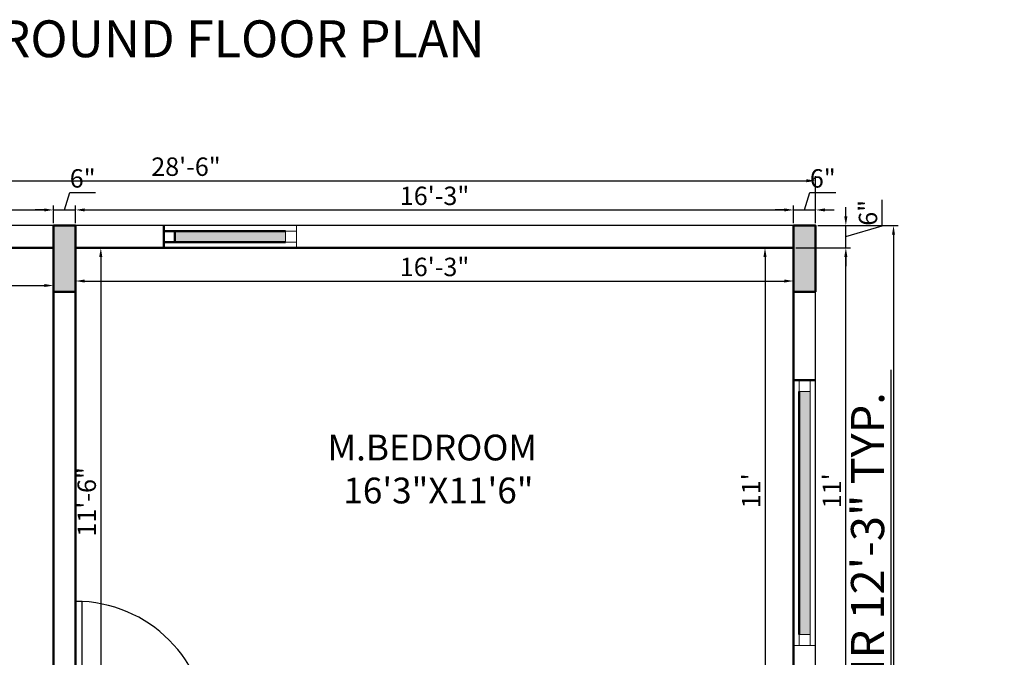
# Model space of a CAD drawing. Units: inches. Extents: x 3064 to 19385, y 846 to 15425.
# Tile 52 of 108: x 6168 to 6436, y 1279 to 1452. Entities that reach past the tile are written whole.
import ezdxf

# ---------------------------------------------------------------- set-up
doc = ezdxf.new("R2010")
doc.units = ezdxf.units.IN
for name, color, linetype, lineweight in [('A-ANNO-DIMS', 2, 'Continuous', 18), ('A-ANNO-TEXT', 7, 'Continuous', 25), ('A-AREA-IDEN', 3, 'Continuous', 18), ('A-COLS', 1, 'Continuous', 35), ('A-DOOR', 3, 'Continuous', 25), ('A-GLAZ', 4, 'Continuous', 18), ('A-WALL', 7, 'Continuous', 50), ('C-PROP', 6, 'Continuous', 25)]:
    doc.layers.add(name, color=color, linetype=linetype, lineweight=lineweight)
doc.styles.get("Standard").update_dxf_attribs({"font": 'arial.ttf'})
doc.dimstyles.new('ISO-25', dxfattribs={"dimtxt": 9, "dimasz": 2.5, "dimexe": 1.25, "dimexo": 0.625, "dimtad": 1, "dimdec": 1, "dimlunit": 3, "dimtxsty": 'Standard', "dimcen": 2.5, "dimadec": 0, "dimazin": 0, "dimtfac": 1, "dimtdec": 1, "dimtmove": 0, "dimatfit": 3, "dimfxl": 1, "dimarcsym": 0})

# ---------------------------------------------------------------- blocks, each defined once
blk = doc.blocks.new('*U3')
for p, q in [((0, 0), (0, -6)), ((36, 0), (36, -6))]:
    blk.add_line(p, q)
blk.add_lwpolyline([(0, 0), (0, 36), (1.75, 36), (1.75, 0)], close=True)
blk.add_arc((0, 0), 36, 0, 90)
blk = doc.blocks.new('*D141')
at = {"layer": 'A-ANNO-DIMS', "color": 0, "lineweight": -2, "transparency": 16777216}
for p, q in [((6048.49, 1396.96), (6048.49, 1401.84)), ((6177.49, 1396.96), (6177.49, 1401.84)), ((6050.99, 1400.59), (6174.99, 1400.59))]:
    blk.add_line(p, q, dxfattribs=at)
at = {"layer": 'A-ANNO-DIMS', "color": 0, "transparency": 16777216}
for points in [[(6050.99, 1401.01), (6050.99, 1400.18), (6048.49, 1400.59)], [(6174.99, 1401.01), (6174.99, 1400.18), (6177.49, 1400.59)]]:
    blk.add_solid(points, dxfattribs=at)
at = {"layer": 'Defpoints', "color": 0, "transparency": 16777216}
for p in [(6177.49, 1400.59), (6048.49, 1396.34), (6177.49, 1396.34)]:
    blk.add_point(p, dxfattribs=at)
at = {"layer": 'A-ANNO-DIMS', "color": 0, "transparency": 16777216, "insert": (6112.99, 1403.77), "char_height": 5, "attachment_point": 5}
blk.add_mtext('10\'-9"', dxfattribs=at)
blk = doc.blocks.new('*D142')
at = {"layer": 'A-ANNO-DIMS', "color": 0, "lineweight": -2, "transparency": 16777216}
for p, q in [((6180.49, 1400.59), (6181.91, 1405.33)), ((6181.91, 1405.33), (6188.94, 1405.33)), ((6177.49, 1396.96), (6177.49, 1401.84)), ((6183.49, 1396.96), (6183.49, 1401.84)), ((6174.99, 1400.59), (6172.49, 1400.59)), ((6177.49, 1400.59), (6183.49, 1400.59)), ((6177.49, 1400.59), (6183.49, 1400.59)), ((6185.99, 1400.59), (6188.49, 1400.59))]:
    blk.add_line(p, q, dxfattribs=at)
at = {"layer": 'A-ANNO-DIMS', "color": 0, "transparency": 16777216}
for points in [[(6174.99, 1401.01), (6174.99, 1400.18), (6177.49, 1400.59)], [(6185.99, 1401.01), (6185.99, 1400.18), (6183.49, 1400.59)]]:
    blk.add_solid(points, dxfattribs=at)
at = {"layer": 'Defpoints', "color": 0, "transparency": 16777216}
for p in [(6183.49, 1400.59), (6177.49, 1396.34), (6183.49, 1396.34)]:
    blk.add_point(p, dxfattribs=at)
at = {"layer": 'A-ANNO-DIMS', "color": 0, "transparency": 16777216, "insert": (6185.43, 1408.51), "char_height": 5, "attachment_point": 5}
blk.add_mtext('6"', dxfattribs=at)
blk = doc.blocks.new('*D143')
at = {"layer": 'A-ANNO-DIMS', "color": 0, "lineweight": -2, "transparency": 16777216}
for p, q in [((6183.49, 1396.96), (6183.49, 1401.84)), ((6378.49, 1396.96), (6378.49, 1401.84)), ((6185.99, 1400.59), (6375.99, 1400.59))]:
    blk.add_line(p, q, dxfattribs=at)
at = {"layer": 'A-ANNO-DIMS', "color": 0, "transparency": 16777216}
for points in [[(6185.99, 1401.01), (6185.99, 1400.18), (6183.49, 1400.59)], [(6375.99, 1401.01), (6375.99, 1400.18), (6378.49, 1400.59)]]:
    blk.add_solid(points, dxfattribs=at)
at = {"layer": 'Defpoints', "color": 0, "transparency": 16777216}
for p in [(6378.49, 1400.59), (6183.49, 1396.34), (6378.49, 1396.34)]:
    blk.add_point(p, dxfattribs=at)
at = {"layer": 'A-ANNO-DIMS', "color": 0, "transparency": 16777216, "insert": (6280.99, 1403.77), "char_height": 5, "attachment_point": 5}
blk.add_mtext('16\'-3"', dxfattribs=at)
blk = doc.blocks.new('*D144')
at = {"layer": 'A-ANNO-DIMS', "color": 0, "lineweight": -2, "transparency": 16777216}
for p, q in [((6381.49, 1400.59), (6382.91, 1405.33)), ((6382.91, 1405.33), (6389.94, 1405.33)), ((6378.49, 1396.96), (6378.49, 1401.84)), ((6384.49, 1396.96), (6384.49, 1401.84)), ((6375.99, 1400.59), (6373.49, 1400.59)), ((6378.49, 1400.59), (6384.49, 1400.59)), ((6378.49, 1400.59), (6384.49, 1400.59)), ((6386.99, 1400.59), (6389.49, 1400.59))]:
    blk.add_line(p, q, dxfattribs=at)
at = {"layer": 'A-ANNO-DIMS', "color": 0, "transparency": 16777216}
for points in [[(6375.99, 1401.01), (6375.99, 1400.18), (6378.49, 1400.59)], [(6386.99, 1401.01), (6386.99, 1400.18), (6384.49, 1400.59)]]:
    blk.add_solid(points, dxfattribs=at)
at = {"layer": 'Defpoints', "color": 0, "transparency": 16777216}
for p in [(6384.49, 1400.59), (6378.49, 1396.34), (6384.49, 1396.34)]:
    blk.add_point(p, dxfattribs=at)
at = {"layer": 'A-ANNO-DIMS', "color": 0, "transparency": 16777216, "insert": (6386.43, 1408.51), "char_height": 5, "attachment_point": 5}
blk.add_mtext('6"', dxfattribs=at)
blk = doc.blocks.new('*D131')
at = {"layer": 'A-ANNO-DIMS', "color": 0, "lineweight": -2, "transparency": 16777216}
for p, q in [((6379.12, 1390.34), (6393.94, 1390.34)), ((6392.69, 1260.84), (6392.69, 1387.84)), ((6385.12, 1258.34), (6393.94, 1258.34))]:
    blk.add_line(p, q, dxfattribs=at)
at = {"layer": 'A-ANNO-DIMS', "color": 0, "transparency": 16777216}
for points in [[(6392.27, 1387.84), (6393.1, 1387.84), (6392.69, 1390.34)], [(6392.27, 1260.84), (6393.1, 1260.84), (6392.69, 1258.34)]]:
    blk.add_solid(points, dxfattribs=at)
at = {"layer": 'Defpoints', "color": 0, "transparency": 16777216}
for p in [(6378.49, 1390.34), (6392.69, 1390.34), (6384.49, 1258.34)]:
    blk.add_point(p, dxfattribs=at)
at = {"layer": 'A-ANNO-DIMS', "color": 0, "transparency": 16777216, "insert": (6389.55, 1324.34), "char_height": 5, "attachment_point": 5, "rotation": 90}
blk.add_mtext("11'", dxfattribs=at)
blk = doc.blocks.new('*D132')
at = {"layer": 'A-ANNO-DIMS', "color": 0, "lineweight": -2, "transparency": 16777216}
for p, q in [((6392.69, 1398.84), (6392.69, 1401.34)), ((6402.53, 1396.29), (6402.53, 1403.32)), ((6385.12, 1396.34), (6393.94, 1396.34)), ((6392.69, 1390.34), (6392.69, 1396.34)), ((6392.69, 1390.34), (6392.69, 1396.34)), ((6392.69, 1393.34), (6402.53, 1396.29)), ((6379.12, 1390.34), (6393.94, 1390.34)), ((6392.69, 1387.84), (6392.69, 1385.34))]:
    blk.add_line(p, q, dxfattribs=at)
at = {"layer": 'A-ANNO-DIMS', "color": 0, "transparency": 16777216}
for points in [[(6392.27, 1398.84), (6393.1, 1398.84), (6392.69, 1396.34)], [(6392.27, 1387.84), (6393.1, 1387.84), (6392.69, 1390.34)]]:
    blk.add_solid(points, dxfattribs=at)
at = {"layer": 'Defpoints', "color": 0, "transparency": 16777216}
for p in [(6384.49, 1396.34), (6392.69, 1396.34), (6378.49, 1390.34)]:
    blk.add_point(p, dxfattribs=at)
at = {"layer": 'A-ANNO-DIMS', "color": 0, "transparency": 16777216, "insert": (6399.35, 1399.81), "char_height": 5, "attachment_point": 5, "rotation": 90}
blk.add_mtext('6"', dxfattribs=at)
blk = doc.blocks.new('*D133')
at = {"layer": 'A-ANNO-DIMS', "color": 0, "lineweight": -2, "transparency": 16777216}
for p, q in [((6385.12, 1396.34), (6406.89, 1396.34)), ((6405.64, 1393.84), (6405.64, 882.84)), ((6385.12, 880.34), (6406.89, 880.34))]:
    blk.add_line(p, q, dxfattribs=at)
at = {"layer": 'A-ANNO-DIMS', "color": 0, "transparency": 16777216}
for points in [[(6405.22, 1393.84), (6406.05, 1393.84), (6405.64, 1396.34)], [(6405.22, 882.84), (6406.05, 882.84), (6405.64, 880.34)]]:
    blk.add_solid(points, dxfattribs=at)
at = {"layer": 'Defpoints', "color": 0, "transparency": 16777216}
for p in [(6384.49, 1396.34), (6384.49, 880.34), (6405.64, 880.34)]:
    blk.add_point(p, dxfattribs=at)
at = {"layer": 'A-ANNO-DIMS', "color": 0, "transparency": 16777216, "insert": (6402.46, 1138.34), "char_height": 5, "attachment_point": 5, "rotation": 90}
blk.add_mtext("43'", dxfattribs=at)
blk = doc.blocks.new('*D134')
at = {"layer": 'A-ANNO-DIMS', "color": 0, "lineweight": -2, "transparency": 16777216}
for p, q in [((6042.49, 1396.96), (6042.49, 1409.76)), ((6384.49, 1396.96), (6384.49, 1409.76)), ((6044.99, 1408.51), (6381.99, 1408.51))]:
    blk.add_line(p, q, dxfattribs=at)
at = {"layer": 'A-ANNO-DIMS', "color": 0, "transparency": 16777216}
for points in [[(6044.99, 1408.93), (6044.99, 1408.1), (6042.49, 1408.51)], [(6381.99, 1408.93), (6381.99, 1408.1), (6384.49, 1408.51)]]:
    blk.add_solid(points, dxfattribs=at)
at = {"layer": 'Defpoints', "color": 0, "transparency": 16777216}
for p in [(6384.49, 1408.51), (6042.49, 1396.34), (6384.49, 1396.34)]:
    blk.add_point(p, dxfattribs=at)
at = {"layer": 'A-ANNO-DIMS', "color": 0, "transparency": 16777216, "insert": (6213.49, 1411.69), "char_height": 5, "attachment_point": 5}
blk.add_mtext('28\'-6"', dxfattribs=at)
blk = doc.blocks.new('*D148')
at = {"layer": 'A-ANNO-DIMS', "color": 0, "lineweight": -2, "transparency": 16777216}
for p, q in [((6048.49, 1389.71), (6048.49, 1378.82)), ((6177.49, 1389.71), (6177.49, 1378.82)), ((6050.99, 1380.07), (6174.99, 1380.07))]:
    blk.add_line(p, q, dxfattribs=at)
at = {"layer": 'A-ANNO-DIMS', "color": 0, "transparency": 16777216}
for points in [[(6050.99, 1380.49), (6050.99, 1379.66), (6048.49, 1380.07)], [(6174.99, 1380.49), (6174.99, 1379.66), (6177.49, 1380.07)]]:
    blk.add_solid(points, dxfattribs=at)
at = {"layer": 'Defpoints', "color": 0, "transparency": 16777216}
for p in [(6048.49, 1390.34), (6177.49, 1390.34), (6177.49, 1380.07)]:
    blk.add_point(p, dxfattribs=at)
at = {"layer": 'A-ANNO-DIMS', "color": 0, "transparency": 16777216, "insert": (6112.99, 1383.25), "char_height": 5, "attachment_point": 5}
blk.add_mtext('10\'-9"', dxfattribs=at)
blk = doc.blocks.new('*D150')
at = {"layer": 'A-ANNO-DIMS', "color": 0, "lineweight": -2, "transparency": 16777216}
for p, q in [((6183.49, 1389.71), (6183.49, 1380.04)), ((6378.49, 1389.71), (6378.49, 1380.04)), ((6185.99, 1381.29), (6375.99, 1381.29))]:
    blk.add_line(p, q, dxfattribs=at)
at = {"layer": 'A-ANNO-DIMS', "color": 0, "transparency": 16777216}
for points in [[(6185.99, 1381.71), (6185.99, 1380.87), (6183.49, 1381.29)], [(6375.99, 1381.71), (6375.99, 1380.87), (6378.49, 1381.29)]]:
    blk.add_solid(points, dxfattribs=at)
at = {"layer": 'Defpoints', "color": 0, "transparency": 16777216}
for p in [(6183.49, 1390.34), (6378.49, 1390.34), (6378.49, 1381.29)]:
    blk.add_point(p, dxfattribs=at)
at = {"layer": 'A-ANNO-DIMS', "color": 0, "transparency": 16777216, "insert": (6280.99, 1384.47), "char_height": 5, "attachment_point": 5}
blk.add_mtext('16\'-3"', dxfattribs=at)
blk = doc.blocks.new('*D151')
at = {"layer": 'A-ANNO-DIMS', "color": 0, "lineweight": -2, "transparency": 16777216}
for p, q in [((6377.87, 1390.34), (6369.49, 1390.34)), ((6370.74, 1387.84), (6370.74, 1260.84)), ((6377.87, 1258.34), (6369.49, 1258.34))]:
    blk.add_line(p, q, dxfattribs=at)
at = {"layer": 'A-ANNO-DIMS', "color": 0, "transparency": 16777216}
for points in [[(6370.32, 1387.84), (6371.16, 1387.84), (6370.74, 1390.34)], [(6370.32, 1260.84), (6371.16, 1260.84), (6370.74, 1258.34)]]:
    blk.add_solid(points, dxfattribs=at)
at = {"layer": 'Defpoints', "color": 0, "transparency": 16777216}
for p in [(6378.49, 1390.34), (6370.74, 1258.34), (6378.49, 1258.34)]:
    blk.add_point(p, dxfattribs=at)
at = {"layer": 'A-ANNO-DIMS', "color": 0, "transparency": 16777216, "insert": (6367.61, 1324.34), "char_height": 5, "attachment_point": 5, "rotation": 90}
blk.add_mtext("11'", dxfattribs=at)
blk = doc.blocks.new('*D156')
at = {"layer": 'A-ANNO-DIMS', "color": 0, "lineweight": -2, "transparency": 16777216}
for p, q in [((6184.12, 1390.34), (6191.61, 1390.34)), ((6190.36, 1387.84), (6190.36, 1254.84)), ((6184.12, 1252.34), (6191.61, 1252.34))]:
    blk.add_line(p, q, dxfattribs=at)
at = {"layer": 'A-ANNO-DIMS', "color": 0, "transparency": 16777216}
for points in [[(6189.94, 1387.84), (6190.77, 1387.84), (6190.36, 1390.34)], [(6189.94, 1254.84), (6190.77, 1254.84), (6190.36, 1252.34)]]:
    blk.add_solid(points, dxfattribs=at)
at = {"layer": 'Defpoints', "color": 0, "transparency": 16777216}
for p in [(6183.49, 1390.34), (6183.49, 1252.34), (6190.36, 1252.34)]:
    blk.add_point(p, dxfattribs=at)
at = {"layer": 'A-ANNO-DIMS', "color": 0, "transparency": 16777216, "insert": (6187.18, 1321.34), "char_height": 5, "attachment_point": 5, "rotation": 90}
blk.add_mtext('11\'-6"', dxfattribs=at)
blk = doc.blocks.new('WIN-1900')
blk.add_line((3, 0), (3, 66))
blk.add_lwpolyline([(3, 66), (0, 66), (0, 69), (3, 69)], close=True)
blk = doc.blocks.new('*D445')
at = {"layer": 'A-ANNO-DIMS', "color": 0, "lineweight": -2, "transparency": 16777216}
for p, q in [((6405.04, 1156.34), (6405.04, 1357.14)), ((6383.62, 1156.34), (6406.29, 1156.34)), ((6405.04, 1011.84), (6405.04, 1153.84)), ((6383.62, 1009.34), (6406.29, 1009.34))]:
    blk.add_line(p, q, dxfattribs=at)
at = {"layer": 'A-ANNO-DIMS', "color": 0, "transparency": 16777216}
for points in [[(6404.63, 1153.84), (6405.46, 1153.84), (6405.04, 1156.34)], [(6404.63, 1011.84), (6405.46, 1011.84), (6405.04, 1009.34)]]:
    blk.add_solid(points, dxfattribs=at)
at = {"layer": 'Defpoints', "color": 0, "transparency": 16777216}
for p in [(6382.99, 1156.34), (6405.04, 1156.34), (6382.99, 1009.34)]:
    blk.add_point(p, dxfattribs=at)
at = {"layer": 'A-ANNO-DIMS', "color": 0, "transparency": 16777216, "insert": (6399.76, 1257.99), "char_height": 9, "attachment_point": 5, "rotation": 90}
blk.add_mtext('WINDOW W1800 PAIR 12\'-3" TYP.', dxfattribs=at)

msp = doc.modelspace()

# ---------------------------------------------------------------- hatches: boundary and pattern name
at = {"layer": 'A-COLS'}
h = msp.add_hatch(color=256, dxfattribs=at)
h.dxf.hatch_style = 1
h.paths.add_polyline_path([(6177.49, 1378.34), (6183.49, 1378.34), (6183.49, 1396.34), (6177.49, 1396.34)])
h = msp.add_hatch(color=256, dxfattribs=at)
h.dxf.hatch_style = 1
h.paths.add_polyline_path([(6378.49, 1378.34), (6384.49, 1378.34), (6384.49, 1396.34), (6378.49, 1396.34)])
at = {"layer": 'A-GLAZ'}
h = msp.add_hatch(color=256, dxfattribs=at)
h.dxf.hatch_style = 1
h.paths.add_polyline_path([(6240.49, 1394.84), (6210.49, 1394.84), (6210.49, 1391.84), (6240.49, 1391.84)])
h = msp.add_hatch(color=256, dxfattribs=at)
h.dxf.hatch_style = 1
h.paths.add_polyline_path([(6379.99, 1285.34), (6382.99, 1285.34), (6382.99, 1351.34), (6379.99, 1351.34)])

# ---------------------------------------------------------------- linework, layer by layer
for p, q in [((6243.49, 1396.34), (6243.49, 1390.34)), ((6384.49, 1282.34), (6378.49, 1282.34))]:
    msp.add_line(p, q, dxfattribs=at)
for points in [[(6243.49, 1391.84), (6240.49, 1391.84), (6240.49, 1394.84), (6243.49, 1394.84)], [(6382.99, 1282.34), (6379.99, 1282.34), (6379.99, 1285.34), (6382.99, 1285.34)]]:
    msp.add_lwpolyline(points, close=True, dxfattribs=at)
at = {"layer": 'A-WALL'}
for p, q in [((6207.49, 1396.34), (6207.49, 1390.34)), ((6210.49, 1394.84), (6240.49, 1394.84)), ((6210.49, 1391.84), (6240.49, 1391.84)), ((6177.49, 1390.34), (6048.49, 1390.34)), ((6177.49, 1390.34), (6177.49, 1252.34)), ((6378.49, 1390.34), (6183.49, 1390.34)), ((6183.49, 1390.34), (6183.49, 1252.34)), ((6378.49, 1258.34), (6378.49, 1390.34)), ((6378.49, 1354.34), (6384.49, 1354.34)), ((6379.99, 1351.34), (6379.99, 1285.34))]:
    msp.add_line(p, q, dxfattribs=at)
for points in [[(6183.49, 1378.34), (6183.49, 1396.34), (6177.49, 1396.34), (6177.49, 1378.34)], [(6384.49, 1378.34), (6384.49, 1396.34), (6378.49, 1396.34), (6378.49, 1378.34)], [(6210.49, 1391.84), (6207.49, 1391.84), (6207.49, 1394.84), (6210.49, 1394.84)]]:
    msp.add_lwpolyline(points, close=True, dxfattribs=at)
at = {"layer": 'C-PROP'}
for p, q in [((6384.49, 1396.34), (6042.49, 1396.34)), ((6384.49, 880.34), (6384.49, 1396.34))]:
    msp.add_line(p, q, dxfattribs=at)

# ---------------------------------------------------------------- block references
at = {"layer": 'A-DOOR'}
msp.add_blockref('*U3', (6183.49, 1258.34), dxfattribs=at)
at = {"layer": 'A-GLAZ'}
msp.add_blockref('WIN-1900', (6379.99, 1285.34), dxfattribs=at)

# ---------------------------------------------------------------- texts
at = {"layer": 'A-ANNO-TEXT', "insert": (6153.16, 1452.06), "char_height": 10, "attachment_point": 1}
msp.add_mtext_dynamic_manual_height_columns('GROUND FLOOR PLAN', width=200.9739, gutter_width=12.5, heights=[0], dxfattribs=at)
at = {"layer": 'A-AREA-IDEN', "insert": (6251.94, 1339.59), "char_height": 7, "attachment_point": 1}
msp.add_mtext_dynamic_manual_height_columns('M.BEDROOM\\P  16\'3"X11\'6"', width=67.5924, gutter_width=12.5, heights=[0], dxfattribs=at)

# ---------------------------------------------------------------- dimensions: what is measured, and where the dimension line sits
at = {"layer": 'A-ANNO-DIMS'}
for base, p1, p2, override, picture, middle in [((6384.49, 1408.51), (6042.49, 1396.34), (6384.49, 1396.34), {"dimtxt": 5, "dimclrd": 0, "dimclre": 0, "dimclrt": 0}, '*D134', (6213.49, 1411.69)), ((6183.49, 1400.59), (6177.49, 1396.34), (6183.49, 1396.34), {"dimtxt": 5, "dimclrd": 0, "dimclre": 0, "dimclrt": 0, "dimtmove": 1}, '*D142', (6182.54, 1408.51)), ((6384.49, 1400.59), (6378.49, 1396.34), (6384.49, 1396.34), {"dimtxt": 5, "dimclrd": 0, "dimclre": 0, "dimclrt": 0, "dimtmove": 1}, '*D144', (6383.54, 1408.51)), ((6177.49, 1400.59), (6048.49, 1396.34), (6177.49, 1396.34), {"dimtxt": 5, "dimclrd": 0, "dimclre": 0, "dimclrt": 0, "dimtmove": 1}, '*D141', (6112.99, 1403.77)), ((6378.49, 1400.59), (6183.49, 1396.34), (6378.49, 1396.34), {"dimtxt": 5, "dimclrd": 0, "dimclre": 0, "dimclrt": 0, "dimtmove": 1}, '*D143', (6280.99, 1403.77)), ((6177.49, 1380.07), (6048.49, 1390.34), (6177.49, 1390.34), {"dimtxt": 5, "dimclrd": 0, "dimclre": 0, "dimclrt": 0}, '*D148', (6112.99, 1383.25)), ((6378.49, 1381.29), (6183.49, 1390.34), (6378.49, 1390.34), {"dimtxt": 5, "dimclrd": 0, "dimclre": 0, "dimclrt": 0}, '*D150', (6280.99, 1384.47))]:
    dim = msp.add_linear_dim(base=base, p1=p1, p2=p2, dimstyle='ISO-25', override=override, dxfattribs=at)
    dim.commit()
    dim.dimension.update_dxf_attribs({"geometry": picture, "text_midpoint": middle})
for base, p1, p2, override, picture, middle in [((6392.69, 1396.34), (6378.49, 1390.34), (6384.49, 1396.34), {"dimtxt": 5, "dimclrd": 0, "dimclre": 0, "dimclrt": 0, "dimtmove": 1}, '*D132', (6399.35, 1396.92)), ((6405.64, 880.34), (6384.49, 1396.34), (6384.49, 880.34), {"dimtxt": 5, "dimclrd": 0, "dimclre": 0, "dimclrt": 0}, '*D133', (6402.46, 1138.34)), ((6190.36, 1252.34), (6183.49, 1390.34), (6183.49, 1252.34), {"dimtxt": 5, "dimclrd": 0, "dimclre": 0, "dimclrt": 0}, '*D156', (6187.18, 1321.34)), ((6370.74, 1258.34), (6378.49, 1390.34), (6378.49, 1258.34), {"dimtxt": 5, "dimclrd": 0, "dimclre": 0, "dimclrt": 0}, '*D151', (6367.61, 1324.34)), ((6392.69, 1390.34), (6384.49, 1258.34), (6378.49, 1390.34), {"dimtxt": 5, "dimclrd": 0, "dimclre": 0, "dimclrt": 0, "dimtmove": 1}, '*D131', (6389.55, 1324.34))]:
    dim = msp.add_linear_dim(base=base, p1=p1, p2=p2, angle=90, dimstyle='ISO-25', override=override, dxfattribs=at)
    dim.commit()
    dim.dimension.update_dxf_attribs({"geometry": picture, "text_midpoint": middle})
dim = msp.add_linear_dim(base=(6405.04, 1156.34), p1=(6382.99, 1009.34), p2=(6382.99, 1156.34), angle=90, text='WINDOW W1800 PAIR <> TYP.', dimstyle='ISO-25', override={"dimdec": 1, "dimrnd": 0, "dimzin": 1, "dimlunit": 4, "dimfrac": 2}, dxfattribs=at)
dim.commit()
dim.dimension.update_dxf_attribs({"geometry": '*D445', "text_midpoint": (6399.76, 1257.99)})

doc.saveas('drawing.dxf')
